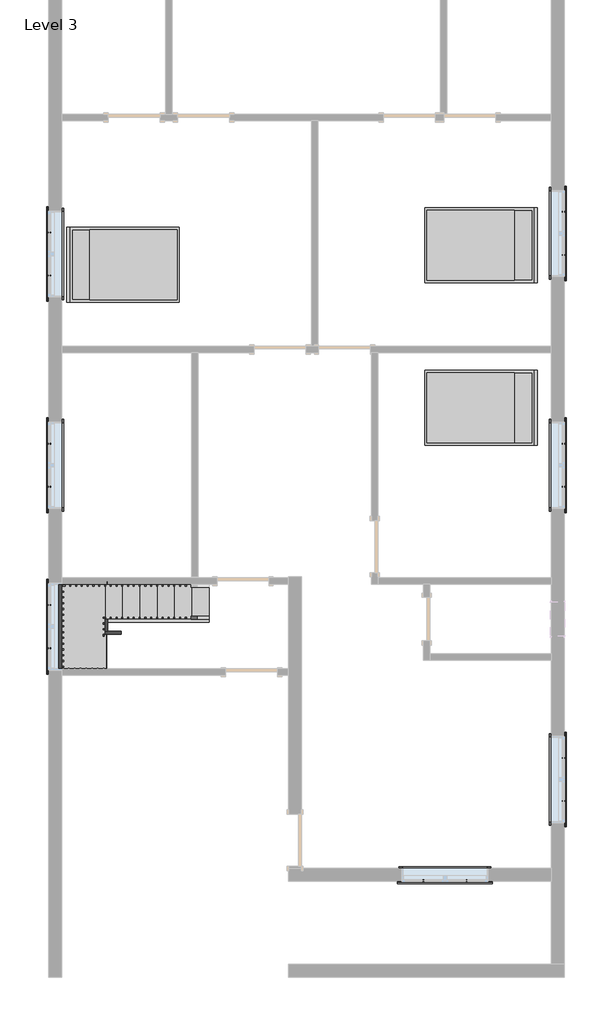
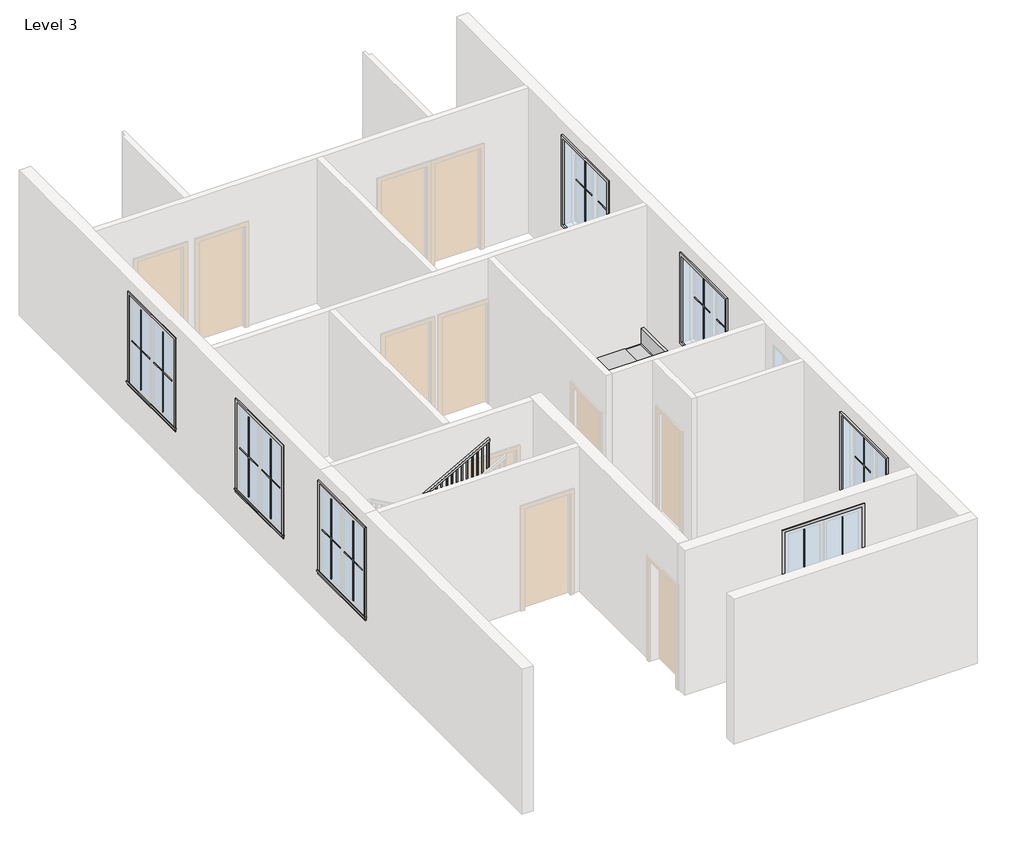
# One storey, part 3 of 3: 28 proxies, 6 members, 3 furniture elements, 1 railing, 1 stair flight.
"""IFC4 building model written with IfcOpenShell, lengths in millimetres."""

from ifc_helpers import new_model, si_unit, frame, origin, place, context, project, spatial, polyline, outline, extrude, faceted_brep, transform, mapped, element, save
from components import muntin_pattern_2x2_muntin_pattern_2x2_f6a80940, muntin_pattern_2x2_muntin_pattern_2x2_09b00a1c, trim_window_exterior_flat_with_sill_698ed857, trim_window_interior_flat_picture_frame_92551a5e, bed_17739_bed_17739_15c61121, stair_flight_b71cab51

model = new_model("IFC4")

# Units and contexts
model_context = context("Model", 3, world=origin())
ifc_project = project(units=[si_unit("LENGTHUNIT", "METRE", prefix="MILLI")], contexts=[model_context])

# Site, building, storey
site = spatial("IfcSite", under=ifc_project)
building = spatial("IfcBuilding", under=site)
storey = spatial("IfcBuildingStorey", under=building, Name="Level 3", Elevation=3200.4)

# Proxies
placement = place(None, origin())
muntin_pattern_2x2_muntin_pattern_2x2_shape = muntin_pattern_2x2_muntin_pattern_2x2_f6a80940(model_context)
element("IfcBuildingElementProxy", 1, Name="Muntin Pattern_2x2 : Muntin Pattern_2x2", ObjectType="Muntin Pattern_2x2 : Muntin Pattern_2x2", at=placement, inside=storey, context=model_context, shape_type="MappedRepresentation", body=[
    mapped(muntin_pattern_2x2_muntin_pattern_2x2_shape, transform((-5778.6870155, 3260.8309309, 4184.65), x_axis=(0.0, 1.0, 0.0), y_axis=(-1.0, 0.0, 0.0), z_axis=(0.0, 0.0, 1.0))),
])
element("IfcBuildingElementProxy", 2, Name="Muntin Pattern_2x2 : Muntin Pattern_2x2", ObjectType="Muntin Pattern_2x2 : Muntin Pattern_2x2", at=placement, inside=storey, context=model_context, shape_type="MappedRepresentation", body=[
    mapped(muntin_pattern_2x2_muntin_pattern_2x2_shape, transform((3270.0629845, 4381.6059309, 4184.65), x_axis=(0.0, -1.0, 0.0), y_axis=(1.0, 0.0, 0.0), z_axis=(0.0, 0.0, 1.0))),
])
element("IfcBuildingElementProxy", 3, Name="Muntin Pattern_2x2 : Muntin Pattern_2x2", ObjectType="Muntin Pattern_2x2 : Muntin Pattern_2x2", at=placement, inside=storey, context=model_context, shape_type="MappedRepresentation", body=[
    mapped(muntin_pattern_2x2_muntin_pattern_2x2_shape, transform((3270.0629845, 304.9059309, 4184.65), x_axis=(0.0, -1.0, 0.0), y_axis=(1.0, 0.0, 0.0), z_axis=(0.0, 0.0, 1.0))),
])
element("IfcBuildingElementProxy", 4, Name="Muntin Pattern_2x2 : Muntin Pattern_2x2", ObjectType="Muntin Pattern_2x2 : Muntin Pattern_2x2", at=placement, inside=storey, context=model_context, shape_type="MappedRepresentation", body=[
    mapped(muntin_pattern_2x2_muntin_pattern_2x2_shape, transform((3270.0629845, -5219.5940691, 4184.65), x_axis=(0.0, -1.0, 0.0), y_axis=(1.0, 0.0, 0.0), z_axis=(0.0, 0.0, 1.0))),
])
element("IfcBuildingElementProxy", 5, Name="Muntin Pattern_2x2 : Muntin Pattern_2x2", ObjectType="Muntin Pattern_2x2 : Muntin Pattern_2x2", at=placement, inside=storey, context=model_context, shape_type="MappedRepresentation", body=[
    mapped(muntin_pattern_2x2_muntin_pattern_2x2_shape, transform((1563.5004845, -7380.1815691, 4184.65), x_axis=(-1.0, 0.0, 0.0), y_axis=(0.0, -1.0, 0.0), z_axis=(0.0, 0.0, 1.0))),
])
element("IfcBuildingElementProxy", 6, Name="Muntin Pattern_2x2 : Muntin Pattern_2x2", ObjectType="Muntin Pattern_2x2 : Muntin Pattern_2x2", at=placement, inside=storey, context=model_context, shape_type="MappedRepresentation", body=[
    mapped(muntin_pattern_2x2_muntin_pattern_2x2_shape, transform((-5778.6870155, -3292.3690691, 4184.65), x_axis=(0.0, 1.0, 0.0), y_axis=(-1.0, 0.0, 0.0), z_axis=(0.0, 0.0, 1.0))),
])
element("IfcBuildingElementProxy", 7, Name="Muntin Pattern_2x2 : Muntin Pattern_2x2", ObjectType="Muntin Pattern_2x2 : Muntin Pattern_2x2", at=placement, inside=storey, context=model_context, shape_type="MappedRepresentation", body=[
    mapped(muntin_pattern_2x2_muntin_pattern_2x2_shape, transform((-5778.6870155, -453.9190691, 4184.65), x_axis=(0.0, 1.0, 0.0), y_axis=(-1.0, 0.0, 0.0), z_axis=(0.0, 0.0, 1.0))),
])
muntin_pattern_2x2_muntin_pattern_2x2_2_shape = muntin_pattern_2x2_muntin_pattern_2x2_09b00a1c(model_context)
element("IfcBuildingElementProxy", 8, Name="Muntin Pattern_2x2 : Muntin Pattern_2x2", ObjectType="Muntin Pattern_2x2 : Muntin Pattern_2x2", at=placement, inside=storey, context=model_context, shape_type="MappedRepresentation", body=[
    mapped(muntin_pattern_2x2_muntin_pattern_2x2_2_shape, transform((-5778.6870155, 4019.6559309, 4184.65), x_axis=(0.0, -1.0, 0.0), y_axis=(1.0, 0.0, 0.0), z_axis=(0.0, 0.0, 1.0))),
])
element("IfcBuildingElementProxy", 9, Name="Muntin Pattern_2x2 : Muntin Pattern_2x2", ObjectType="Muntin Pattern_2x2 : Muntin Pattern_2x2", at=placement, inside=storey, context=model_context, shape_type="MappedRepresentation", body=[
    mapped(muntin_pattern_2x2_muntin_pattern_2x2_2_shape, transform((3270.0629845, 3622.7809309, 4184.65), x_axis=(0.0, 1.0, 0.0), y_axis=(-1.0, 0.0, 0.0), z_axis=(0.0, 0.0, 1.0))),
])
element("IfcBuildingElementProxy", 10, Name="Muntin Pattern_2x2 : Muntin Pattern_2x2", ObjectType="Muntin Pattern_2x2 : Muntin Pattern_2x2", at=placement, inside=storey, context=model_context, shape_type="MappedRepresentation", body=[
    mapped(muntin_pattern_2x2_muntin_pattern_2x2_2_shape, transform((3270.0629845, -453.9190691, 4184.65), x_axis=(0.0, 1.0, 0.0), y_axis=(-1.0, 0.0, 0.0), z_axis=(0.0, 0.0, 1.0))),
])
element("IfcBuildingElementProxy", 11, Name="Muntin Pattern_2x2 : Muntin Pattern_2x2", ObjectType="Muntin Pattern_2x2 : Muntin Pattern_2x2", at=placement, inside=storey, context=model_context, shape_type="MappedRepresentation", body=[
    mapped(muntin_pattern_2x2_muntin_pattern_2x2_2_shape, transform((3270.0629845, -5978.4190691, 4184.65), x_axis=(0.0, 1.0, 0.0), y_axis=(-1.0, 0.0, 0.0), z_axis=(0.0, 0.0, 1.0))),
])
element("IfcBuildingElementProxy", 12, Name="Muntin Pattern_2x2 : Muntin Pattern_2x2", ObjectType="Muntin Pattern_2x2 : Muntin Pattern_2x2", at=placement, inside=storey, context=model_context, shape_type="MappedRepresentation", body=[
    mapped(muntin_pattern_2x2_muntin_pattern_2x2_2_shape, transform((804.6754845, -7380.1815691, 4184.65), x_axis=(1.0, 0.0, 0.0), y_axis=(0.0, 1.0, 0.0), z_axis=(0.0, 0.0, 1.0))),
])
element("IfcBuildingElementProxy", 13, Name="Muntin Pattern_2x2 : Muntin Pattern_2x2", ObjectType="Muntin Pattern_2x2 : Muntin Pattern_2x2", at=placement, inside=storey, context=model_context, shape_type="MappedRepresentation", body=[
    mapped(muntin_pattern_2x2_muntin_pattern_2x2_2_shape, transform((-5778.6870155, -2533.5440691, 4184.65), x_axis=(0.0, -1.0, 0.0), y_axis=(1.0, 0.0, 0.0), z_axis=(0.0, 0.0, 1.0))),
])
element("IfcBuildingElementProxy", 14, Name="Muntin Pattern_2x2 : Muntin Pattern_2x2", ObjectType="Muntin Pattern_2x2 : Muntin Pattern_2x2", at=placement, inside=storey, context=model_context, shape_type="MappedRepresentation", body=[
    mapped(muntin_pattern_2x2_muntin_pattern_2x2_2_shape, transform((-5778.6870155, 304.9059309, 4184.65), x_axis=(0.0, -1.0, 0.0), y_axis=(1.0, 0.0, 0.0), z_axis=(0.0, 0.0, 1.0))),
])
trim_window_exterior_flat_with_sill_shape = trim_window_exterior_flat_with_sill_698ed857(model_context)
element("IfcBuildingElementProxy", 15, Name="Trim-Window-Exterior-Flat : with Sill", ObjectType="Trim-Window-Exterior-Flat : with Sill", at=placement, inside=storey, context=model_context, shape_type="MappedRepresentation", body=[
    mapped(trim_window_exterior_flat_with_sill_shape, transform((-5788.2120155, 3640.2434309, 5943.6), x_axis=(0.0, -1.0, 0.0), y_axis=(0.0, 0.0, 1.0), z_axis=(-1.0, 0.0, 0.0))),
])
element("IfcBuildingElementProxy", 16, Name="Trim-Window-Exterior-Flat : with Sill", ObjectType="Trim-Window-Exterior-Flat : with Sill", at=placement, inside=storey, context=model_context, shape_type="MappedRepresentation", body=[
    mapped(trim_window_exterior_flat_with_sill_shape, transform((3279.5879845, 4002.1934309, 5943.6), x_axis=(0.0, 1.0, 0.0), y_axis=(0.0, 0.0, 1.0), z_axis=(1.0, 0.0, 0.0))),
])
element("IfcBuildingElementProxy", 17, Name="Trim-Window-Exterior-Flat : with Sill", ObjectType="Trim-Window-Exterior-Flat : with Sill", at=placement, inside=storey, context=model_context, shape_type="MappedRepresentation", body=[
    mapped(trim_window_exterior_flat_with_sill_shape, transform((3279.5879845, -74.5065691, 5943.6), x_axis=(0.0, 1.0, 0.0), y_axis=(0.0, 0.0, 1.0), z_axis=(1.0, 0.0, 0.0))),
])
element("IfcBuildingElementProxy", 18, Name="Trim-Window-Exterior-Flat : with Sill", ObjectType="Trim-Window-Exterior-Flat : with Sill", at=placement, inside=storey, context=model_context, shape_type="MappedRepresentation", body=[
    mapped(trim_window_exterior_flat_with_sill_shape, transform((3279.5879845, -5599.0065691, 5943.6), x_axis=(0.0, 1.0, 0.0), y_axis=(0.0, 0.0, 1.0), z_axis=(1.0, 0.0, 0.0))),
])
element("IfcBuildingElementProxy", 19, Name="Trim-Window-Exterior-Flat : with Sill", ObjectType="Trim-Window-Exterior-Flat : with Sill", at=placement, inside=storey, context=model_context, shape_type="MappedRepresentation", body=[
    mapped(trim_window_exterior_flat_with_sill_shape, transform((1184.0879845, -7389.7065691, 5943.6), x_axis=(1.0, 0.0, 0.0), y_axis=(0.0, 0.0, 1.0), z_axis=(0.0, -1.0, 0.0))),
])
element("IfcBuildingElementProxy", 20, Name="Trim-Window-Exterior-Flat : with Sill", ObjectType="Trim-Window-Exterior-Flat : with Sill", at=placement, inside=storey, context=model_context, shape_type="MappedRepresentation", body=[
    mapped(trim_window_exterior_flat_with_sill_shape, transform((-5788.2120155, -2912.9565691, 5943.6), x_axis=(0.0, -1.0, 0.0), y_axis=(0.0, 0.0, 1.0), z_axis=(-1.0, 0.0, 0.0))),
])
element("IfcBuildingElementProxy", 21, Name="Trim-Window-Exterior-Flat : with Sill", ObjectType="Trim-Window-Exterior-Flat : with Sill", at=placement, inside=storey, context=model_context, shape_type="MappedRepresentation", body=[
    mapped(trim_window_exterior_flat_with_sill_shape, transform((-5788.2120155, -74.5065691, 5943.6), x_axis=(0.0, -1.0, 0.0), y_axis=(0.0, 0.0, 1.0), z_axis=(-1.0, 0.0, 0.0))),
])
trim_window_interior_flat_picture_frame_shape = trim_window_interior_flat_picture_frame_92551a5e(model_context)
element("IfcBuildingElementProxy", 22, Name="Trim-Window-Interior-Flat : Picture Frame", ObjectType="Trim-Window-Interior-Flat : Picture Frame", at=placement, inside=storey, context=model_context, shape_type="MappedRepresentation", body=[
    mapped(trim_window_interior_flat_picture_frame_shape, transform((-5559.6120155, 3640.2434309, 5943.6), x_axis=(0.0, 1.0, 0.0), y_axis=(0.0, 0.0, 1.0), z_axis=(1.0, 0.0, 0.0))),
])
element("IfcBuildingElementProxy", 23, Name="Trim-Window-Interior-Flat : Picture Frame", ObjectType="Trim-Window-Interior-Flat : Picture Frame", at=placement, inside=storey, context=model_context, shape_type="MappedRepresentation", body=[
    mapped(trim_window_interior_flat_picture_frame_shape, transform((3050.9879845, 4002.1934309, 5943.6), x_axis=(0.0, -1.0, 0.0), y_axis=(0.0, 0.0, 1.0), z_axis=(-1.0, 0.0, 0.0))),
])
element("IfcBuildingElementProxy", 24, Name="Trim-Window-Interior-Flat : Picture Frame", ObjectType="Trim-Window-Interior-Flat : Picture Frame", at=placement, inside=storey, context=model_context, shape_type="MappedRepresentation", body=[
    mapped(trim_window_interior_flat_picture_frame_shape, transform((3050.9879845, -74.5065691, 5943.6), x_axis=(0.0, -1.0, 0.0), y_axis=(0.0, 0.0, 1.0), z_axis=(-1.0, 0.0, 0.0))),
])
element("IfcBuildingElementProxy", 25, Name="Trim-Window-Interior-Flat : Picture Frame", ObjectType="Trim-Window-Interior-Flat : Picture Frame", at=placement, inside=storey, context=model_context, shape_type="MappedRepresentation", body=[
    mapped(trim_window_interior_flat_picture_frame_shape, transform((3050.9879845, -5599.0065691, 5943.6), x_axis=(0.0, -1.0, 0.0), y_axis=(0.0, 0.0, 1.0), z_axis=(-1.0, 0.0, 0.0))),
])
element("IfcBuildingElementProxy", 26, Name="Trim-Window-Interior-Flat : Picture Frame", ObjectType="Trim-Window-Interior-Flat : Picture Frame", at=placement, inside=storey, context=model_context, shape_type="MappedRepresentation", body=[
    mapped(trim_window_interior_flat_picture_frame_shape, transform((1184.0879845, -7161.1065691, 5943.6), x_axis=(-1.0, 0.0, 0.0), y_axis=(0.0, 0.0, 1.0), z_axis=(0.0, 1.0, 0.0))),
])
element("IfcBuildingElementProxy", 27, Name="Trim-Window-Interior-Flat : Picture Frame", ObjectType="Trim-Window-Interior-Flat : Picture Frame", at=placement, inside=storey, context=model_context, shape_type="MappedRepresentation", body=[
    mapped(trim_window_interior_flat_picture_frame_shape, transform((-5559.6120155, -2912.9565691, 5943.6), x_axis=(0.0, 1.0, 0.0), y_axis=(0.0, 0.0, 1.0), z_axis=(1.0, 0.0, 0.0))),
])
element("IfcBuildingElementProxy", 28, Name="Trim-Window-Interior-Flat : Picture Frame", ObjectType="Trim-Window-Interior-Flat : Picture Frame", at=placement, inside=storey, context=model_context, shape_type="MappedRepresentation", body=[
    mapped(trim_window_interior_flat_picture_frame_shape, transform((-5559.6120155, -74.5065691, 5943.6), x_axis=(0.0, 1.0, 0.0), y_axis=(0.0, 0.0, 1.0), z_axis=(1.0, 0.0, 0.0))),
])

# Furniture
bed_17739_bed_17739_shape = bed_17739_bed_17739_15c61121(model_context)
element("IfcFurniture", 29, ObjectType="Bed_17739 : Bed_17739", at=placement, inside=storey, context=model_context, shape_type="MappedRepresentation", body=[
    mapped(bed_17739_bed_17739_shape, transform((-4454.7120155, 3449.7434309, 3200.4), x_axis=(0.0, 1.0, 0.0), y_axis=(-1.0, 0.0, 0.0), z_axis=(0.0, 0.0, 1.0))),
])
element("IfcFurniture", 30, ObjectType="Bed_17739 : Bed_17739", at=placement, inside=storey, context=model_context, shape_type="MappedRepresentation", body=[
    mapped(bed_17739_bed_17739_shape, transform((1793.6879845, 3792.6434309, 3200.4), x_axis=(0.0, -1.0, 0.0), y_axis=(1.0, 0.0, 0.0), z_axis=(0.0, 0.0, 1.0))),
])
element("IfcFurniture", 31, ObjectType="Bed_17739 : Bed_17739", at=placement, inside=storey, context=model_context, shape_type="MappedRepresentation", body=[
    mapped(bed_17739_bed_17739_shape, transform((1793.6879845, 935.1434309, 3200.4), x_axis=(0.0, -1.0, 0.0), y_axis=(1.0, 0.0, 0.0), z_axis=(0.0, 0.0, 1.0))),
])

# Members
element("IfcMember", 32, ObjectType="Stringer - 2\" Width", at=placement, inside=storey, context=model_context, shape_type="SweptSolid", body=[
    extrude(outline(polyline([(3200.4, -2968.8120155), (3407.9983948, -2968.8120155), (4395.7761726, -4746.8120155), (4047.0974984, -4746.8120155), (3200.4, -3222.7565183), (3200.4, -2968.8120155)])), frame((0.0, -2830.4065691, 0.0), z_axis=(0.0, 1.0, 0.0), x_axis=(0.0, 0.0, 1.0)), (0.0, 0.0, 1.0), 50.8),
])
element("IfcMember", 33, ObjectType="Stringer - 2\" Width", at=placement, inside=storey, context=model_context, shape_type="SweptSolid", body=[
    extrude(outline(polyline([(-4797.6120155, -2779.6065691), (-4746.8120155, -2779.6065691), (-4746.8120155, -2995.5065691), (-4797.6120155, -2995.5065691), (-4797.6120155, -2779.6065691)])), frame((0.0, 0.0, 4157.1333333), z_axis=(0.0, 0.0, 1.0), x_axis=(1.0, 0.0, 0.0)), (0.0, 0.0, 1.0), 304.8),
])
element("IfcMember", 34, ObjectType="Stringer - 2\" Width", at=placement, inside=storey, context=model_context, shape_type="SweptSolid", body=[
    extrude(outline(polyline([(4593.3317281, -4797.6120155), (4244.653054, -4797.6120155), (5260.653054, -2968.8120155), (5609.3317281, -2968.8120155), (4593.3317281, -4797.6120155)])), frame((0.0, -3046.3065691, 0.0), z_axis=(0.0, 1.0, 0.0), x_axis=(0.0, 0.0, 1.0)), (0.0, 0.0, 1.0), 50.8),
])
element("IfcMember", 35, ObjectType="Stringer - 2\" Width", at=placement, inside=storey, context=model_context, shape_type="SweptSolid", body=[
    extrude(outline(polyline([(3200.4, -2968.8120155), (3407.9983948, -2968.8120155), (4461.9333333, -4865.8949049), (4461.9333333, -5493.5165183), (3200.4, -3222.7565183), (3200.4, -2968.8120155)])), frame((0.0, -2170.0065691, 0.0), z_axis=(0.0, 1.0, 0.0), x_axis=(0.0, 0.0, 1.0)), (0.0, 0.0, 1.0), 50.8),
])
element("IfcMember", 36, ObjectType="Stringer - 2\" Width", at=placement, inside=storey, context=model_context, shape_type="SweptSolid", body=[
    extrude(outline(polyline([(-5610.4120155, -2119.2065691), (-5559.6120155, -2119.2065691), (-5559.6120155, -3674.9565691), (-5610.4120155, -3674.9565691), (-5610.4120155, -2119.2065691)])), frame((0.0, 0.0, 4157.1333333), z_axis=(0.0, 0.0, 1.0), x_axis=(1.0, 0.0, 0.0)), (0.0, 0.0, 1.0), 304.8),
])
element("IfcMember", 37, ObjectType="Stringer - 2\" Width", at=placement, inside=storey, context=model_context, shape_type="SweptSolid", body=[
    extrude(outline(polyline([(4157.1333333, -4955.1475127), (5260.653054, -2968.8120155), (5609.3317281, -2968.8120155), (4157.1333333, -5582.7691261), (4157.1333333, -4955.1475127)])), frame((0.0, -3725.7565691, 0.0), z_axis=(0.0, 1.0, 0.0), x_axis=(0.0, 0.0, 1.0)), (0.0, 0.0, 1.0), 50.8),
])

# Railing
element("IfcRailing", 38, ObjectType="Handrail - Rectangular", at=placement, inside=storey, context=model_context, shape_type="SolidModel", body=[
    faceted_brep([(-2968.8120155, -2779.6065691, 4284.1333333), (-2968.8120155, -2779.6065691, 4226.020221), (-2968.8120155, -2728.8065691, 4226.020221), (-2968.8120155, -2728.8065691, 4284.1333333), (-4721.4120155, -2779.6065691, 5257.8), (-4772.2120155, -2779.6065691, 5227.9091099), (-4772.2120155, -2728.8065691, 5227.9091099), (-4721.4120155, -2728.8065691, 5257.8), (-4721.4120155, -2779.6065691, 5300.1333333), (-4772.2120155, -2779.6065691, 5249.3333333), (-4772.2120155, -2728.8065691, 5249.3333333), (-4721.4120155, -2728.8065691, 5300.1333333), (-4797.6120155, -2779.6065691, 5300.1333333), (-4797.6120155, -2779.6065691, 5249.3333333), (-4848.4120155, -2728.8065691, 5249.3333333), (-4848.4120155, -2728.8065691, 5300.1333333), (-4797.6120155, -2855.8065691, 5300.1333333), (-4797.6120155, -2855.8065691, 5249.3333333), (-4848.4120155, -2855.8065691, 5249.3333333), (-4848.4120155, -2855.8065691, 5300.1333333), (-4797.6120155, -2970.1065691, 5300.1333333), (-4797.6120155, -3020.9065691, 5249.3333333), (-4848.4120155, -3020.9065691, 5249.3333333), (-4848.4120155, -2970.1065691, 5300.1333333), (-4797.6120155, -2970.1065691, 5511.8), (-4797.6120155, -3020.9065691, 5461.0), (-4848.4120155, -3020.9065691, 5461.0), (-4848.4120155, -2970.1065691, 5511.8), (-4797.6120155, -3046.3065691, 5511.8), (-4797.6120155, -3046.3065691, 5461.0), (-4848.4120155, -3097.1065691, 5461.0), (-4848.4120155, -3097.1065691, 5511.8), (-4721.4120155, -3046.3065691, 5511.8), (-4708.2484132, -3046.3065691, 5461.0), (-4708.2484132, -3097.1065691, 5461.0), (-4721.4120155, -3097.1065691, 5511.8), (-2968.8120155, -3046.3065691, 6485.4666667), (-2968.8120155, -3097.1065691, 6485.4666667), (-2968.8120155, -3097.1065691, 6427.3535543), (-2968.8120155, -3046.3065691, 6427.3535543)], [[[0, 1, 2, 3]], [[1, 0, 4, 5]], [[2, 1, 5, 6]], [[3, 2, 6, 7]], [[0, 3, 7, 4]], [[5, 4, 8, 9]], [[6, 5, 9, 10]], [[7, 6, 10, 11]], [[4, 7, 11, 8]], [[9, 8, 12, 13]], [[10, 9, 13, 14]], [[11, 10, 14, 15]], [[8, 11, 15, 12]], [[13, 12, 16, 17]], [[14, 13, 17, 18]], [[15, 14, 18, 19]], [[12, 15, 19, 16]], [[17, 16, 20, 21]], [[18, 17, 21, 22]], [[19, 18, 22, 23]], [[16, 19, 23, 20]], [[21, 20, 24, 25]], [[22, 21, 25, 26]], [[23, 22, 26, 27]], [[20, 23, 27, 24]], [[25, 24, 28, 29]], [[26, 25, 29, 30]], [[27, 26, 30, 31]], [[24, 27, 31, 28]], [[29, 28, 32, 33]], [[30, 29, 33, 34]], [[31, 30, 34, 35]], [[28, 31, 35, 32]], [[36, 37, 38, 39]], [[33, 32, 36, 39]], [[34, 33, 39, 38]], [[35, 34, 38, 37]], [[32, 35, 37, 36]]]),
    extrude(outline(polyline([(6407.9507765, -3003.7370155), (5401.7333333, -3003.7370155), (5401.7333333, -2984.6870155), (6418.5341099, -2984.6870155), (6407.9507765, -3003.7370155)])), frame((0.0, -3081.2315691, 0.0), z_axis=(0.0, 1.0, 0.0), x_axis=(0.0, 0.0, 1.0)), (0.0, 0.0, 1.0), 19.05),
    extrude(outline(polyline([(6351.5063321, -3105.3370155), (5401.7333333, -3105.3370155), (5401.7333333, -3086.2870155), (6362.0896654, -3086.2870155), (6351.5063321, -3105.3370155)])), frame((0.0, -3081.2315691, 0.0), z_axis=(0.0, 1.0, 0.0), x_axis=(0.0, 0.0, 1.0)), (0.0, 0.0, 1.0), 19.05),
    extrude(outline(polyline([(6295.0618876, -3206.9370155), (5401.7333333, -3206.9370155), (5401.7333333, -3187.8870155), (6305.645221, -3187.8870155), (6295.0618876, -3206.9370155)])), frame((0.0, -3081.2315691, 0.0), z_axis=(0.0, 1.0, 0.0), x_axis=(0.0, 0.0, 1.0)), (0.0, 0.0, 1.0), 19.05),
    extrude(outline(polyline([(6238.6174432, -3308.5370155), (5232.4, -3308.5370155), (5232.4, -3289.4870155), (6249.2007765, -3289.4870155), (6238.6174432, -3308.5370155)])), frame((0.0, -3081.2315691, 0.0), z_axis=(0.0, 1.0, 0.0), x_axis=(0.0, 0.0, 1.0)), (0.0, 0.0, 1.0), 19.05),
    extrude(outline(polyline([(6182.1729988, -3410.1370155), (5232.4, -3410.1370155), (5232.4, -3391.0870155), (6192.7563321, -3391.0870155), (6182.1729988, -3410.1370155)])), frame((0.0, -3081.2315691, 0.0), z_axis=(0.0, 1.0, 0.0), x_axis=(0.0, 0.0, 1.0)), (0.0, 0.0, 1.0), 19.05),
    extrude(outline(polyline([(6125.7285543, -3511.7370155), (5232.4, -3511.7370155), (5232.4, -3492.6870155), (6136.3118876, -3492.6870155), (6125.7285543, -3511.7370155)])), frame((0.0, -3081.2315691, 0.0), z_axis=(0.0, 1.0, 0.0), x_axis=(0.0, 0.0, 1.0)), (0.0, 0.0, 1.0), 19.05),
    extrude(outline(polyline([(6069.2841099, -3613.3370155), (5063.0666667, -3613.3370155), (5063.0666667, -3594.2870155), (6079.8674432, -3594.2870155), (6069.2841099, -3613.3370155)])), frame((0.0, -3081.2315691, 0.0), z_axis=(0.0, 1.0, 0.0), x_axis=(0.0, 0.0, 1.0)), (0.0, 0.0, 1.0), 19.05),
    extrude(outline(polyline([(6012.8396654, -3714.9370155), (5063.0666667, -3714.9370155), (5063.0666667, -3695.8870155), (6023.4229988, -3695.8870155), (6012.8396654, -3714.9370155)])), frame((0.0, -3081.2315691, 0.0), z_axis=(0.0, 1.0, 0.0), x_axis=(0.0, 0.0, 1.0)), (0.0, 0.0, 1.0), 19.05),
    extrude(outline(polyline([(5956.395221, -3816.5370155), (5063.0666667, -3816.5370155), (5063.0666667, -3797.4870155), (5966.9785543, -3797.4870155), (5956.395221, -3816.5370155)])), frame((0.0, -3081.2315691, 0.0), z_axis=(0.0, 1.0, 0.0), x_axis=(0.0, 0.0, 1.0)), (0.0, 0.0, 1.0), 19.05),
    extrude(outline(polyline([(5899.9507765, -3918.1370155), (4893.7333333, -3918.1370155), (4893.7333333, -3899.0870155), (5910.5341099, -3899.0870155), (5899.9507765, -3918.1370155)])), frame((0.0, -3081.2315691, 0.0), z_axis=(0.0, 1.0, 0.0), x_axis=(0.0, 0.0, 1.0)), (0.0, 0.0, 1.0), 19.05),
    extrude(outline(polyline([(5843.5063321, -4019.7370155), (4893.7333333, -4019.7370155), (4893.7333333, -4000.6870155), (5854.0896654, -4000.6870155), (5843.5063321, -4019.7370155)])), frame((0.0, -3081.2315691, 0.0), z_axis=(0.0, 1.0, 0.0), x_axis=(0.0, 0.0, 1.0)), (0.0, 0.0, 1.0), 19.05),
    extrude(outline(polyline([(5787.0618876, -4121.3370155), (4893.7333333, -4121.3370155), (4893.7333333, -4102.2870155), (5797.645221, -4102.2870155), (5787.0618876, -4121.3370155)])), frame((0.0, -3081.2315691, 0.0), z_axis=(0.0, 1.0, 0.0), x_axis=(0.0, 0.0, 1.0)), (0.0, 0.0, 1.0), 19.05),
    extrude(outline(polyline([(5730.6174432, -4222.9370155), (4724.4, -4222.9370155), (4724.4, -4203.8870155), (5741.2007765, -4203.8870155), (5730.6174432, -4222.9370155)])), frame((0.0, -3081.2315691, 0.0), z_axis=(0.0, 1.0, 0.0), x_axis=(0.0, 0.0, 1.0)), (0.0, 0.0, 1.0), 19.05),
    extrude(outline(polyline([(5674.1729988, -4324.5370155), (4724.4, -4324.5370155), (4724.4, -4305.4870155), (5684.7563321, -4305.4870155), (5674.1729988, -4324.5370155)])), frame((0.0, -3081.2315691, 0.0), z_axis=(0.0, 1.0, 0.0), x_axis=(0.0, 0.0, 1.0)), (0.0, 0.0, 1.0), 19.05),
    extrude(outline(polyline([(5617.7285543, -4426.1370155), (4724.4, -4426.1370155), (4724.4, -4407.0870155), (5628.3118876, -4407.0870155), (5617.7285543, -4426.1370155)])), frame((0.0, -3081.2315691, 0.0), z_axis=(0.0, 1.0, 0.0), x_axis=(0.0, 0.0, 1.0)), (0.0, 0.0, 1.0), 19.05),
    extrude(outline(polyline([(5561.2841099, -4527.7370155), (4555.0666667, -4527.7370155), (4555.0666667, -4508.6870155), (5571.8674432, -4508.6870155), (5561.2841099, -4527.7370155)])), frame((0.0, -3081.2315691, 0.0), z_axis=(0.0, 1.0, 0.0), x_axis=(0.0, 0.0, 1.0)), (0.0, 0.0, 1.0), 19.05),
    extrude(outline(polyline([(5504.8396654, -4629.3370155), (4555.0666667, -4629.3370155), (4555.0666667, -4610.2870155), (5515.4229988, -4610.2870155), (5504.8396654, -4629.3370155)])), frame((0.0, -3081.2315691, 0.0), z_axis=(0.0, 1.0, 0.0), x_axis=(0.0, 0.0, 1.0)), (0.0, 0.0, 1.0), 19.05),
    extrude(outline(polyline([(5448.395221, -4730.9370155), (4555.0666667, -4730.9370155), (4555.0666667, -4711.8870155), (5458.9785543, -4711.8870155), (5448.395221, -4730.9370155)])), frame((0.0, -3081.2315691, 0.0), z_axis=(0.0, 1.0, 0.0), x_axis=(0.0, 0.0, 1.0)), (0.0, 0.0, 1.0), 19.05),
    extrude(outline(polyline([(-4813.4870155, -3049.4815691), (-4813.4870155, -3068.5315691), (-4832.5370155, -3068.5315691), (-4832.5370155, -3049.4815691), (-4813.4870155, -3049.4815691)])), frame((0.0, 0.0, 4385.7333333), z_axis=(0.0, 0.0, 1.0), x_axis=(1.0, 0.0, 0.0)), (0.0, 0.0, 1.0), 1075.2666667),
    extrude(outline(polyline([(-4813.4870155, -2947.8815691), (-4813.4870155, -2966.9315691), (-4832.5370155, -2966.9315691), (-4832.5370155, -2947.8815691), (-4813.4870155, -2947.8815691)])), frame((0.0, 0.0, 4385.7333333), z_axis=(0.0, 0.0, 1.0), x_axis=(1.0, 0.0, 0.0)), (0.0, 0.0, 1.0), 863.6),
    extrude(outline(polyline([(-4813.4870155, -2846.2815691), (-4813.4870155, -2865.3315691), (-4832.5370155, -2865.3315691), (-4832.5370155, -2846.2815691), (-4813.4870155, -2846.2815691)])), frame((0.0, 0.0, 4385.7333333), z_axis=(0.0, 0.0, 1.0), x_axis=(1.0, 0.0, 0.0)), (0.0, 0.0, 1.0), 863.6),
    extrude(outline(polyline([(-4788.0870155, -2763.7315691), (-4807.1370155, -2763.7315691), (-4807.1370155, -2744.6815691), (-4788.0870155, -2744.6815691), (-4788.0870155, -2763.7315691)])), frame((0.0, 0.0, 4385.7333333), z_axis=(0.0, 0.0, 1.0), x_axis=(1.0, 0.0, 0.0)), (0.0, 0.0, 1.0), 863.6),
    extrude(outline(polyline([(5190.8674432, -4705.5370155), (4216.4, -4705.5370155), (4216.4, -4686.4870155), (5180.2841099, -4686.4870155), (5190.8674432, -4705.5370155)])), frame((0.0, -2763.7315691, 0.0), z_axis=(0.0, 1.0, 0.0), x_axis=(0.0, 0.0, 1.0)), (0.0, 0.0, 1.0), 19.05),
    extrude(outline(polyline([(5134.4229988, -4603.9370155), (4216.4, -4603.9370155), (4216.4, -4584.8870155), (5123.8396654, -4584.8870155), (5134.4229988, -4603.9370155)])), frame((0.0, -2763.7315691, 0.0), z_axis=(0.0, 1.0, 0.0), x_axis=(0.0, 0.0, 1.0)), (0.0, 0.0, 1.0), 19.05),
    extrude(outline(polyline([(5077.9785543, -4502.3370155), (4216.4, -4502.3370155), (4216.4, -4483.2870155), (5067.395221, -4483.2870155), (5077.9785543, -4502.3370155)])), frame((0.0, -2763.7315691, 0.0), z_axis=(0.0, 1.0, 0.0), x_axis=(0.0, 0.0, 1.0)), (0.0, 0.0, 1.0), 19.05),
    extrude(outline(polyline([(5021.5341099, -4400.7370155), (4047.0666667, -4400.7370155), (4047.0666667, -4381.6870155), (5010.9507765, -4381.6870155), (5021.5341099, -4400.7370155)])), frame((0.0, -2763.7315691, 0.0), z_axis=(0.0, 1.0, 0.0), x_axis=(0.0, 0.0, 1.0)), (0.0, 0.0, 1.0), 19.05),
    extrude(outline(polyline([(4965.0896654, -4299.1370155), (4047.0666667, -4299.1370155), (4047.0666667, -4280.0870155), (4954.5063321, -4280.0870155), (4965.0896654, -4299.1370155)])), frame((0.0, -2763.7315691, 0.0), z_axis=(0.0, 1.0, 0.0), x_axis=(0.0, 0.0, 1.0)), (0.0, 0.0, 1.0), 19.05),
    extrude(outline(polyline([(4908.645221, -4197.5370155), (4047.0666667, -4197.5370155), (4047.0666667, -4178.4870155), (4898.0618876, -4178.4870155), (4908.645221, -4197.5370155)])), frame((0.0, -2763.7315691, 0.0), z_axis=(0.0, 1.0, 0.0), x_axis=(0.0, 0.0, 1.0)), (0.0, 0.0, 1.0), 19.05),
    extrude(outline(polyline([(4852.2007765, -4095.9370155), (3877.7333333, -4095.9370155), (3877.7333333, -4076.8870155), (4841.6174432, -4076.8870155), (4852.2007765, -4095.9370155)])), frame((0.0, -2763.7315691, 0.0), z_axis=(0.0, 1.0, 0.0), x_axis=(0.0, 0.0, 1.0)), (0.0, 0.0, 1.0), 19.05),
    extrude(outline(polyline([(4795.7563321, -3994.3370155), (3877.7333333, -3994.3370155), (3877.7333333, -3975.2870155), (4785.1729988, -3975.2870155), (4795.7563321, -3994.3370155)])), frame((0.0, -2763.7315691, 0.0), z_axis=(0.0, 1.0, 0.0), x_axis=(0.0, 0.0, 1.0)), (0.0, 0.0, 1.0), 19.05),
    extrude(outline(polyline([(4739.3118876, -3892.7370155), (3877.7333333, -3892.7370155), (3877.7333333, -3873.6870155), (4728.7285543, -3873.6870155), (4739.3118876, -3892.7370155)])), frame((0.0, -2763.7315691, 0.0), z_axis=(0.0, 1.0, 0.0), x_axis=(0.0, 0.0, 1.0)), (0.0, 0.0, 1.0), 19.05),
    extrude(outline(polyline([(4682.8674432, -3791.1370155), (3708.4, -3791.1370155), (3708.4, -3772.0870155), (4672.2841099, -3772.0870155), (4682.8674432, -3791.1370155)])), frame((0.0, -2763.7315691, 0.0), z_axis=(0.0, 1.0, 0.0), x_axis=(0.0, 0.0, 1.0)), (0.0, 0.0, 1.0), 19.05),
    extrude(outline(polyline([(4626.4229988, -3689.5370155), (3708.4, -3689.5370155), (3708.4, -3670.4870155), (4615.8396654, -3670.4870155), (4626.4229988, -3689.5370155)])), frame((0.0, -2763.7315691, 0.0), z_axis=(0.0, 1.0, 0.0), x_axis=(0.0, 0.0, 1.0)), (0.0, 0.0, 1.0), 19.05),
    extrude(outline(polyline([(4569.9785543, -3587.9370155), (3708.4, -3587.9370155), (3708.4, -3568.8870155), (4559.395221, -3568.8870155), (4569.9785543, -3587.9370155)])), frame((0.0, -2763.7315691, 0.0), z_axis=(0.0, 1.0, 0.0), x_axis=(0.0, 0.0, 1.0)), (0.0, 0.0, 1.0), 19.05),
    extrude(outline(polyline([(4513.5341099, -3486.3370155), (3539.0666667, -3486.3370155), (3539.0666667, -3467.2870155), (4502.9507765, -3467.2870155), (4513.5341099, -3486.3370155)])), frame((0.0, -2763.7315691, 0.0), z_axis=(0.0, 1.0, 0.0), x_axis=(0.0, 0.0, 1.0)), (0.0, 0.0, 1.0), 19.05),
    extrude(outline(polyline([(4457.0896654, -3384.7370155), (3539.0666667, -3384.7370155), (3539.0666667, -3365.6870155), (4446.5063321, -3365.6870155), (4457.0896654, -3384.7370155)])), frame((0.0, -2763.7315691, 0.0), z_axis=(0.0, 1.0, 0.0), x_axis=(0.0, 0.0, 1.0)), (0.0, 0.0, 1.0), 19.05),
    extrude(outline(polyline([(4400.645221, -3283.1370155), (3539.0666667, -3283.1370155), (3539.0666667, -3264.0870155), (4390.0618876, -3264.0870155), (4400.645221, -3283.1370155)])), frame((0.0, -2763.7315691, 0.0), z_axis=(0.0, 1.0, 0.0), x_axis=(0.0, 0.0, 1.0)), (0.0, 0.0, 1.0), 19.05),
    extrude(outline(polyline([(4344.2007765, -3181.5370155), (3369.7333333, -3181.5370155), (3369.7333333, -3162.4870155), (4333.6174432, -3162.4870155), (4344.2007765, -3181.5370155)])), frame((0.0, -2763.7315691, 0.0), z_axis=(0.0, 1.0, 0.0), x_axis=(0.0, 0.0, 1.0)), (0.0, 0.0, 1.0), 19.05),
    extrude(outline(polyline([(4287.7563321, -3079.9370155), (3369.7333333, -3079.9370155), (3369.7333333, -3060.8870155), (4277.1729988, -3060.8870155), (4287.7563321, -3079.9370155)])), frame((0.0, -2763.7315691, 0.0), z_axis=(0.0, 1.0, 0.0), x_axis=(0.0, 0.0, 1.0)), (0.0, 0.0, 1.0), 19.05),
    extrude(outline(polyline([(-4813.4870155, -3062.1815691), (-4813.4870155, -3081.2315691), (-4832.5370155, -3081.2315691), (-4832.5370155, -3062.1815691), (-4813.4870155, -3062.1815691)])), frame((0.0, 0.0, 4385.7333333), z_axis=(0.0, 0.0, 1.0), x_axis=(1.0, 0.0, 0.0)), (0.0, 0.0, 1.0), 1075.2666667),
    extrude(outline(polyline([(-4813.4870155, -2763.7315691), (-4832.5370155, -2763.7315691), (-4832.5370155, -2744.6815691), (-4813.4870155, -2744.6815691), (-4813.4870155, -2763.7315691)])), frame((0.0, 0.0, 4385.7333333), z_axis=(0.0, 0.0, 1.0), x_axis=(1.0, 0.0, 0.0)), (0.0, 0.0, 1.0), 863.6),
    extrude(outline(polyline([(6416.770221, -2987.8620155), (5401.7333333, -2987.8620155), (5401.7333333, -2968.8120155), (6427.3535543, -2968.8120155), (6416.770221, -2987.8620155)])), frame((0.0, -3081.2315691, 0.0), z_axis=(0.0, 1.0, 0.0), x_axis=(0.0, 0.0, 1.0)), (0.0, 0.0, 1.0), 19.05),
    extrude(outline(polyline([(4236.6035543, -2987.8620155), (3369.7333333, -2987.8620155), (3369.7333333, -2968.8120155), (4226.020221, -2968.8120155), (4236.6035543, -2987.8620155)])), frame((0.0, -2763.7315691, 0.0), z_axis=(0.0, 1.0, 0.0), x_axis=(0.0, 0.0, 1.0)), (0.0, 0.0, 1.0), 19.05),
])

# Stair flight
stair_flight_shape = stair_flight_b71cab51(model_context)
element("IfcStairFlight", 39, ObjectType="2\" Tread 1\" Nosing 1/4\" Riser", at=placement, inside=storey, context=model_context, shape_type="MappedRepresentation", body=[
    mapped(stair_flight_shape, transform((0.0, 0.0, 0.0), x_axis=(1.0, 0.0, 0.0), y_axis=(0.0, 1.0, 0.0), z_axis=(0.0, 0.0, 1.0))),
])

save(model, "model.ifc")

# Revit data of these elements
# Type "Muntin Pattern_2x2 : Muntin Pattern_2x2"
#   Width [instance default] = 4' - 0"
#   Thickness = 0' - 0 1/2"
#   Height [instance default] = 4' - 0"
#   Distance = 0' - 0 3/4"
#   Interior Material [instance default] = none
#   Exterior Material [instance default] = none
#   Default Elevation = 0
# Type "Trim-Window-Exterior-Flat : with Sill"
#   Trim Width = 0' - 2 1/4"
#   Trim Thickness_Picture Frame = 0' - 1 1/4"
#   Trim Thickness_with Sill = 0' - 0 3/4"
#   Sill Thickness = 0' - 1 1/4"
#   Opening Width [instance default] = 2' - 0"
#   Opening Height [instance default] = 3' - 0"
#   Default Elevation = 4' - 0"
#   Sill = yes
#   Picture Frame = no
#   Trim Material [instance default] = none
# Type "Trim-Window-Interior-Flat : Picture Frame"
#   Trim Thickness_Picture Frame = 0' - 1 1/4"
#   Trim Width = 0' - 2 1/4"
#   Trim Thickness_with Sill = 0' - 0 3/4"
#   Sill Thickness = 0' - 1 1/4"
#   Opening Width [instance default] = 2' - 0"
#   Opening Height [instance default] = 3' - 0"
#   Default Elevation = 4' - 0"
#   Sill = no
#   Picture Frame = yes
#   Trim Material [instance default] = none
# Type "Bed_17739 : Bed_17739"
#   Default Elevation = 0
# Type "Handrail - Rectangular"
#   Assembly Code = "C2010400"
#   built-in parameter 1008612 = 0.0416667 (stored number, unit not read)
#   built-in parameter 1008611 = 0.0416667 (stored number, unit not read)
#   built-in parameter 1008609 = 0.333333 (stored number, unit not read)
#   built-in parameter 1008604 = 0.166667 (stored number, unit not read)
#   built-in parameter 1008603 = 0.166667 (stored number, unit not read)
#   Railing Height = 3' - 0"
#   built-in parameter 1008630 = 2
#   built-in parameter 1008610 = 2
#   built-in parameter 1008618 = Baluster - Square : 3/4"
# Elements 1, 2, 3, 4, 5, 6, 7, 8, 9, 10, 11, 12, 13, 14 (IfcBuildingElementProxy, "Muntin Pattern_2x2 : Muntin Pattern_2x2")
#   Width = 2' - 0 5/8"
#   Height = 5' - 6 1/2"
#   Interior Material = Wood - Stained
#   Exterior Material = Clad - White
#   Phase Created = New Construction
#   Materials on its faces: "Clad - White", "Wood - Stained"
# Elements 15, 16, 17, 18, 19, 20, 21 (IfcBuildingElementProxy, "Trim-Window-Exterior-Flat : with Sill")
#   Opening Width = 5' - 0"
#   Opening Height = 6' - 0"
#   Trim Material = Clad - White
#   Phase Created = New Construction
#   Materials on its faces: "Clad - White"
# Elements 22, 23, 24, 25, 26, 27, 28 (IfcBuildingElementProxy, "Trim-Window-Interior-Flat : Picture Frame")
#   Opening Width = 5' - 0"
#   Opening Height = 6' - 0"
#   Trim Material = Wood - Stained
#   Phase Created = New Construction
#   Materials on its faces: "Wood - Stained"
# Elements 29, 30, 31 (IfcFurniture, "Bed_17739 : Bed_17739")
#   Phase Created = New Construction
#   Materials on its faces: "legs", "sheets", "bed frame", "Blanket"
# Elements 32, 33, 34, 35, 36, 37 (IfcMember, "Stringer - 2\" Width")
#   Phase Created = New Construction
# Element 38 (IfcRailing, "Handrail - Rectangular")
#   Phase Created = New Construction
# Element 39 (IfcStairFlight, "2\" Tread 1\" Nosing 1/4\" Riser")
#   Phase Created = New Construction
# Materials
#   "Clad - White": class "Wood", colour RGB 242 242 238, transparency 0, Cost = 0
#   "Wood - Stained": class "Wood", colour RGB 224 178 126, transparency 0, Cost = 0
#   "legs": colour RGB 90 73 37, transparency 0, Cost = 0
#   "sheets": colour RGB 200 195 176, transparency 0, Cost = 0
#   "bed frame": colour RGB 90 73 37, transparency 0, Cost = 0
#   "Blanket": class "System", colour RGB 59 0 1, transparency 0, Cost = 0
